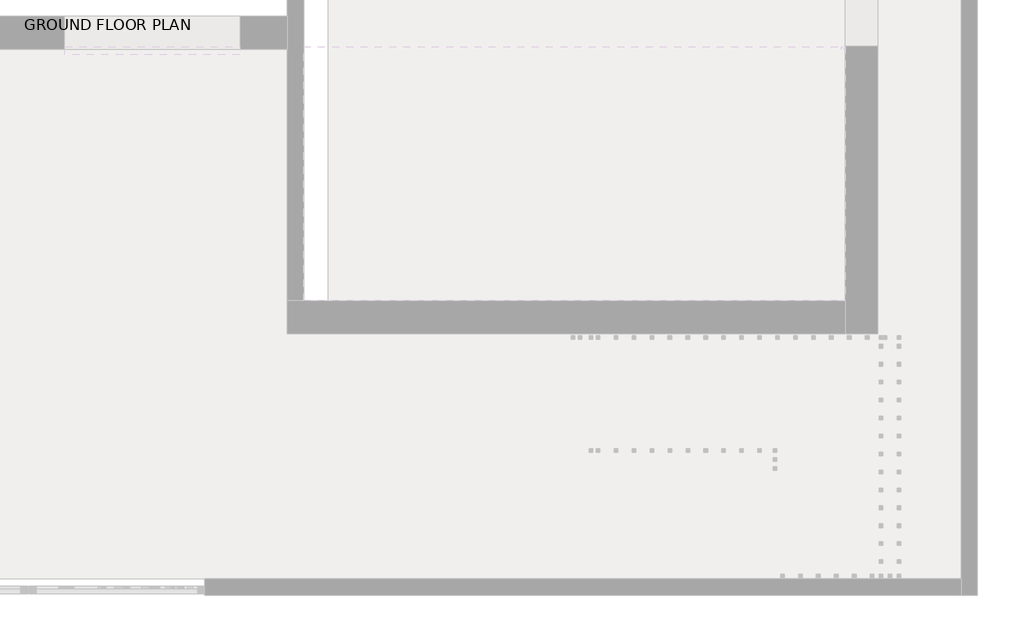
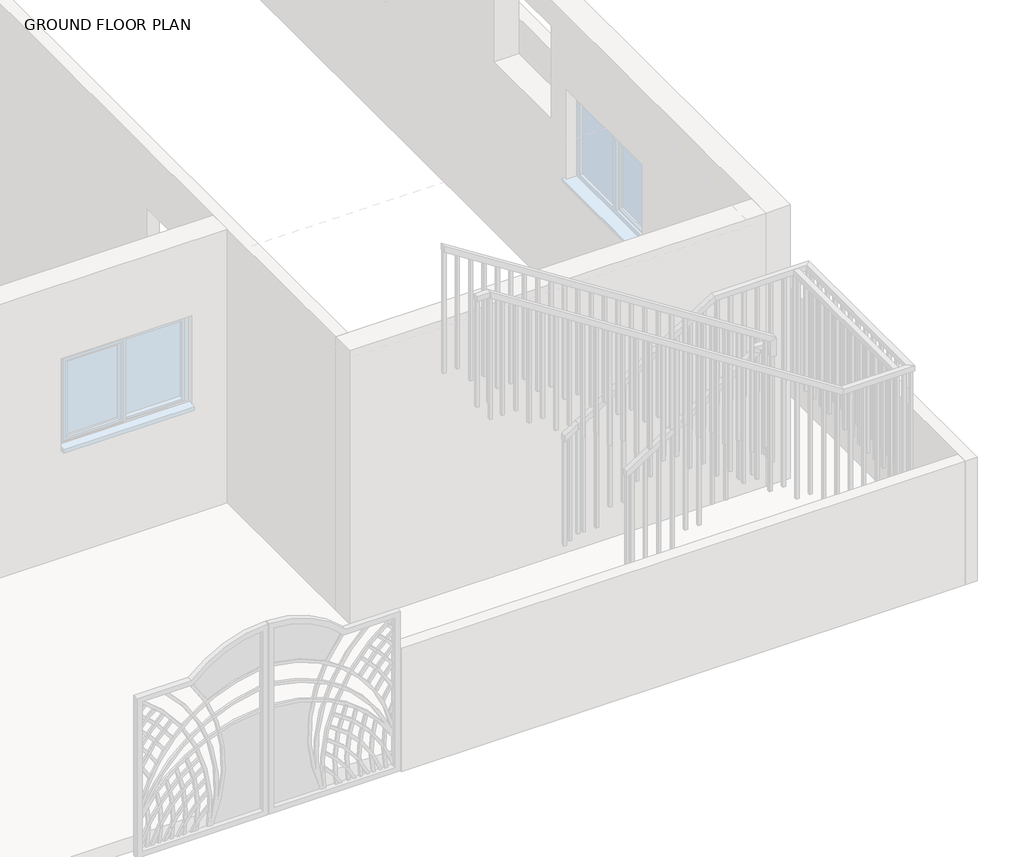
# One storey, part 18 of 23: 2 railings.
"""IFC4 building model written with IfcOpenShell, lengths in millimetres."""

from ifc_helpers import new_model, si_unit, frame, origin, place, context, project, spatial, polyline, outline, extrude, faceted_brep, element, save

model = new_model("IFC4")

# Units and contexts
model_context = context("Model", 3, world=origin())
ifc_project = project(units=[si_unit("LENGTHUNIT", "METRE", prefix="MILLI")], contexts=[model_context])

# Site, building, storey
site = spatial("IfcSite", under=ifc_project)
building = spatial("IfcBuilding", under=site)
storey = spatial("IfcBuildingStorey", under=building, Name="GROUND FLOOR PLAN", Elevation=487.68)

# Railings
placement = place(None, origin())
element("IfcRailing", 1, ObjectType="1100mm", at=placement, inside=storey, context=model_context, shape_type="SolidModel", body=[
    faceted_brep([(-8680.149573, -11007.9255223, 1912.8), (-8680.149573, -11007.9255223, 1853.4423995), (-8680.149573, -11057.9255223, 1853.4423995), (-8680.149573, -11057.9255223, 1912.8), (-7484.3306254, -11007.9255223, 2677.8717446), (-7434.3306254, -11007.9255223, 2650.5035914), (-7434.3306254, -11057.9255223, 2650.5035914), (-7484.3306254, -11057.9255223, 2677.8717446), (-7484.3306254, -11007.9255223, 2725.6), (-7434.3306254, -11007.9255223, 2675.6), (-7434.3306254, -11057.9255223, 2675.6), (-7484.3306254, -11057.9255223, 2725.6), (-7359.3306254, -11007.9255223, 2725.6), (-7359.3306254, -11007.9255223, 2675.6), (-7409.3306254, -11057.9255223, 2675.6), (-7409.3306254, -11057.9255223, 2725.6), (-7359.3306254, -11132.9255223, 2725.6), (-7359.3306254, -11132.9255223, 2675.6), (-7409.3306254, -11132.9255223, 2675.6), (-7409.3306254, -11132.9255223, 2725.6), (-7359.3306254, -11134.9255223, 2725.6), (-7409.3306254, -11134.9255223, 2725.6), (-7409.3306254, -11184.9255223, 2675.6), (-7359.3306254, -11184.9255223, 2675.6)], [[[0, 1, 2, 3]], [[1, 0, 4, 5]], [[2, 1, 5, 6]], [[3, 2, 6, 7]], [[0, 3, 7, 4]], [[5, 4, 8, 9]], [[6, 5, 9, 10]], [[7, 6, 10, 11]], [[4, 7, 11, 8]], [[9, 8, 12, 13]], [[10, 9, 13, 14]], [[11, 10, 14, 15]], [[8, 11, 15, 12]], [[13, 12, 16, 17]], [[14, 13, 17, 18]], [[15, 14, 18, 19]], [[12, 15, 19, 16]], [[20, 21, 22, 23]], [[17, 16, 20, 23]], [[18, 17, 23, 22]], [[19, 18, 22, 21]], [[16, 19, 21, 20]]]),
    faceted_brep([(-7359.3306254, -11184.9255223, 2855.9055527), (-7409.3306254, -11184.9255223, 2828.5415543), (-7409.3306254, -11134.9255223, 2828.5415543), (-7359.3306254, -11134.9255223, 2855.9055527), (-10457.8773536, -11184.9255223, 4838.88), (-10457.8773536, -11134.9255223, 4838.88), (-10457.8773536, -11134.9255223, 4779.517542), (-10457.8773536, -11184.9255223, 4779.517542)], [[[0, 1, 2, 3]], [[4, 5, 6, 7]], [[1, 0, 4, 7]], [[2, 1, 7, 6]], [[3, 2, 6, 5]], [[0, 3, 5, 4]]]),
    faceted_brep([(-7359.3306254, -11134.9255223, 2725.6), (-7359.3306254, -11184.9255223, 2675.6), (-7409.3306254, -11184.9255223, 2675.6), (-7409.3306254, -11134.9255223, 2725.6), (-7359.3306254, -11134.9255223, 2855.9055527), (-7409.3306254, -11134.9255223, 2828.5415543), (-7409.3306254, -11184.9255223, 2828.5415543), (-7359.3306254, -11184.9255223, 2855.9055527)], [[[0, 1, 2, 3]], [[4, 5, 6, 7]], [[1, 0, 4, 7]], [[2, 1, 7, 6]], [[3, 2, 6, 5]], [[0, 3, 5, 4]]]),
    extrude(outline(polyline([(3576.32, -10434.3306254), (4764.4483614, -10434.3306254), (4780.4475912, -10459.3306254), (3576.32, -10459.3306254), (3576.32, -10434.3306254)])), frame((0.0, -11172.4255223, 0.0), z_axis=(0.0, 1.0, 0.0), x_axis=(0.0, 0.0, 1.0)), (0.0, 0.0, 1.0), 25.0),
    extrude(outline(polyline([(3576.32, -10309.3306254), (4684.4522123, -10309.3306254), (4700.4514422, -10334.3306254), (3576.32, -10334.3306254), (3576.32, -10309.3306254)])), frame((0.0, -11172.4255223, 0.0), z_axis=(0.0, 1.0, 0.0), x_axis=(0.0, 0.0, 1.0)), (0.0, 0.0, 1.0), 25.0),
    extrude(outline(polyline([(3413.76, -10184.3306254), (4604.4560633, -10184.3306254), (4620.4552931, -10209.3306254), (3413.76, -10209.3306254), (3413.76, -10184.3306254)])), frame((0.0, -11172.4255223, 0.0), z_axis=(0.0, 1.0, 0.0), x_axis=(0.0, 0.0, 1.0)), (0.0, 0.0, 1.0), 25.0),
    extrude(outline(polyline([(3413.76, -10059.3306254), (4524.4599142, -10059.3306254), (4540.459144, -10084.3306254), (3413.76, -10084.3306254), (3413.76, -10059.3306254)])), frame((0.0, -11172.4255223, 0.0), z_axis=(0.0, 1.0, 0.0), x_axis=(0.0, 0.0, 1.0)), (0.0, 0.0, 1.0), 25.0),
    extrude(outline(polyline([(3251.2, -9934.3306254), (4444.4637652, -9934.3306254), (4460.462995, -9959.3306254), (3251.2, -9959.3306254), (3251.2, -9934.3306254)])), frame((0.0, -11172.4255223, 0.0), z_axis=(0.0, 1.0, 0.0), x_axis=(0.0, 0.0, 1.0)), (0.0, 0.0, 1.0), 25.0),
    extrude(outline(polyline([(3251.2, -9809.3306254), (4364.4676161, -9809.3306254), (4380.4668459, -9834.3306254), (3251.2, -9834.3306254), (3251.2, -9809.3306254)])), frame((0.0, -11172.4255223, 0.0), z_axis=(0.0, 1.0, 0.0), x_axis=(0.0, 0.0, 1.0)), (0.0, 0.0, 1.0), 25.0),
    extrude(outline(polyline([(3251.2, -9684.3306254), (4284.4714671, -9684.3306254), (4300.4706969, -9709.3306254), (3251.2, -9709.3306254), (3251.2, -9684.3306254)])), frame((0.0, -11172.4255223, 0.0), z_axis=(0.0, 1.0, 0.0), x_axis=(0.0, 0.0, 1.0)), (0.0, 0.0, 1.0), 25.0),
    extrude(outline(polyline([(3088.64, -9559.3306254), (4204.475318, -9559.3306254), (4220.4745478, -9584.3306254), (3088.64, -9584.3306254), (3088.64, -9559.3306254)])), frame((0.0, -11172.4255223, 0.0), z_axis=(0.0, 1.0, 0.0), x_axis=(0.0, 0.0, 1.0)), (0.0, 0.0, 1.0), 25.0),
    extrude(outline(polyline([(3088.64, -9434.3306254), (4124.479169, -9434.3306254), (4140.4783988, -9459.3306254), (3088.64, -9459.3306254), (3088.64, -9434.3306254)])), frame((0.0, -11172.4255223, 0.0), z_axis=(0.0, 1.0, 0.0), x_axis=(0.0, 0.0, 1.0)), (0.0, 0.0, 1.0), 25.0),
    extrude(outline(polyline([(2926.08, -9309.3306254), (4044.4830199, -9309.3306254), (4060.4822497, -9334.3306254), (2926.08, -9334.3306254), (2926.08, -9309.3306254)])), frame((0.0, -11172.4255223, 0.0), z_axis=(0.0, 1.0, 0.0), x_axis=(0.0, 0.0, 1.0)), (0.0, 0.0, 1.0), 25.0),
    extrude(outline(polyline([(2926.08, -9184.3306254), (3964.4868709, -9184.3306254), (3980.4861007, -9209.3306254), (2926.08, -9209.3306254), (2926.08, -9184.3306254)])), frame((0.0, -11172.4255223, 0.0), z_axis=(0.0, 1.0, 0.0), x_axis=(0.0, 0.0, 1.0)), (0.0, 0.0, 1.0), 25.0),
    extrude(outline(polyline([(2763.52, -9059.3306254), (3884.4907218, -9059.3306254), (3900.4899516, -9084.3306254), (2763.52, -9084.3306254), (2763.52, -9059.3306254)])), frame((0.0, -11172.4255223, 0.0), z_axis=(0.0, 1.0, 0.0), x_axis=(0.0, 0.0, 1.0)), (0.0, 0.0, 1.0), 25.0),
    extrude(outline(polyline([(2763.52, -8934.3306254), (3804.4945728, -8934.3306254), (3820.4938026, -8959.3306254), (2763.52, -8959.3306254), (2763.52, -8934.3306254)])), frame((0.0, -11172.4255223, 0.0), z_axis=(0.0, 1.0, 0.0), x_axis=(0.0, 0.0, 1.0)), (0.0, 0.0, 1.0), 25.0),
    extrude(outline(polyline([(2600.96, -8809.3306254), (3724.4984237, -8809.3306254), (3740.4976535, -8834.3306254), (2600.96, -8834.3306254), (2600.96, -8809.3306254)])), frame((0.0, -11172.4255223, 0.0), z_axis=(0.0, 1.0, 0.0), x_axis=(0.0, 0.0, 1.0)), (0.0, 0.0, 1.0), 25.0),
    extrude(outline(polyline([(2600.96, -8684.3306254), (3644.5022747, -8684.3306254), (3660.5015045, -8709.3306254), (2600.96, -8709.3306254), (2600.96, -8684.3306254)])), frame((0.0, -11172.4255223, 0.0), z_axis=(0.0, 1.0, 0.0), x_axis=(0.0, 0.0, 1.0)), (0.0, 0.0, 1.0), 25.0),
    extrude(outline(polyline([(2438.4, -8559.3306254), (3564.5061256, -8559.3306254), (3580.5053554, -8584.3306254), (2438.4, -8584.3306254), (2438.4, -8559.3306254)])), frame((0.0, -11172.4255223, 0.0), z_axis=(0.0, 1.0, 0.0), x_axis=(0.0, 0.0, 1.0)), (0.0, 0.0, 1.0), 25.0),
    extrude(outline(polyline([(2438.4, -8434.3306254), (3484.5099766, -8434.3306254), (3500.5092064, -8459.3306254), (2438.4, -8459.3306254), (2438.4, -8434.3306254)])), frame((0.0, -11172.4255223, 0.0), z_axis=(0.0, 1.0, 0.0), x_axis=(0.0, 0.0, 1.0)), (0.0, 0.0, 1.0), 25.0),
    extrude(outline(polyline([(2275.84, -8309.3306254), (3404.5138275, -8309.3306254), (3420.5130573, -8334.3306254), (2275.84, -8334.3306254), (2275.84, -8309.3306254)])), frame((0.0, -11172.4255223, 0.0), z_axis=(0.0, 1.0, 0.0), x_axis=(0.0, 0.0, 1.0)), (0.0, 0.0, 1.0), 25.0),
    extrude(outline(polyline([(2275.84, -8184.3306254), (3324.5176785, -8184.3306254), (3340.5169083, -8209.3306254), (2275.84, -8209.3306254), (2275.84, -8184.3306254)])), frame((0.0, -11172.4255223, 0.0), z_axis=(0.0, 1.0, 0.0), x_axis=(0.0, 0.0, 1.0)), (0.0, 0.0, 1.0), 25.0),
    extrude(outline(polyline([(2113.28, -8059.3306254), (3244.5215294, -8059.3306254), (3260.5207592, -8084.3306254), (2113.28, -8084.3306254), (2113.28, -8059.3306254)])), frame((0.0, -11172.4255223, 0.0), z_axis=(0.0, 1.0, 0.0), x_axis=(0.0, 0.0, 1.0)), (0.0, 0.0, 1.0), 25.0),
    extrude(outline(polyline([(2113.28, -7934.3306254), (3164.5253804, -7934.3306254), (3180.5246102, -7959.3306254), (2113.28, -7959.3306254), (2113.28, -7934.3306254)])), frame((0.0, -11172.4255223, 0.0), z_axis=(0.0, 1.0, 0.0), x_axis=(0.0, 0.0, 1.0)), (0.0, 0.0, 1.0), 25.0),
    extrude(outline(polyline([(1950.72, -7809.3306254), (3084.5292313, -7809.3306254), (3100.5284611, -7834.3306254), (1950.72, -7834.3306254), (1950.72, -7809.3306254)])), frame((0.0, -11172.4255223, 0.0), z_axis=(0.0, 1.0, 0.0), x_axis=(0.0, 0.0, 1.0)), (0.0, 0.0, 1.0), 25.0),
    extrude(outline(polyline([(1950.72, -7684.3306254), (3004.5330823, -7684.3306254), (3020.5323121, -7709.3306254), (1950.72, -7709.3306254), (1950.72, -7684.3306254)])), frame((0.0, -11172.4255223, 0.0), z_axis=(0.0, 1.0, 0.0), x_axis=(0.0, 0.0, 1.0)), (0.0, 0.0, 1.0), 25.0),
    extrude(outline(polyline([(1788.16, -7559.3306254), (2924.5369332, -7559.3306254), (2940.536163, -7584.3306254), (1788.16, -7584.3306254), (1788.16, -7559.3306254)])), frame((0.0, -11172.4255223, 0.0), z_axis=(0.0, 1.0, 0.0), x_axis=(0.0, 0.0, 1.0)), (0.0, 0.0, 1.0), 25.0),
    extrude(outline(polyline([(1788.16, -7434.3306254), (2844.5407841, -7434.3306254), (2860.540014, -7459.3306254), (1788.16, -7459.3306254), (1788.16, -7434.3306254)])), frame((0.0, -11172.4255223, 0.0), z_axis=(0.0, 1.0, 0.0), x_axis=(0.0, 0.0, 1.0)), (0.0, 0.0, 1.0), 25.0),
    extrude(outline(polyline([(-7396.8306254, -11082.9255223), (-7371.8306254, -11082.9255223), (-7371.8306254, -11107.9255223), (-7396.8306254, -11107.9255223), (-7396.8306254, -11082.9255223)])), frame((0.0, 0.0, 1625.6), z_axis=(0.0, 0.0, 1.0), x_axis=(1.0, 0.0, 0.0)), (0.0, 0.0, 1.0), 1050.0),
    extrude(outline(polyline([(2605.1944115, -7505.149573), (1463.04, -7505.149573), (1463.04, -7480.149573), (2621.1891352, -7480.149573), (2605.1944115, -7505.149573)])), frame((0.0, -11045.4255223, 0.0), z_axis=(0.0, 1.0, 0.0), x_axis=(0.0, 0.0, 1.0)), (0.0, 0.0, 1.0), 25.0),
    extrude(outline(polyline([(2525.2207932, -7630.149573), (1463.04, -7630.149573), (1463.04, -7605.149573), (2541.2155169, -7605.149573), (2525.2207932, -7630.149573)])), frame((0.0, -11045.4255223, 0.0), z_axis=(0.0, 1.0, 0.0), x_axis=(0.0, 0.0, 1.0)), (0.0, 0.0, 1.0), 25.0),
    extrude(outline(polyline([(2445.2471749, -7755.149573), (1300.48, -7755.149573), (1300.48, -7730.149573), (2461.2418986, -7730.149573), (2445.2471749, -7755.149573)])), frame((0.0, -11045.4255223, 0.0), z_axis=(0.0, 1.0, 0.0), x_axis=(0.0, 0.0, 1.0)), (0.0, 0.0, 1.0), 25.0),
    extrude(outline(polyline([(2365.2735566, -7880.149573), (1300.48, -7880.149573), (1300.48, -7855.149573), (2381.2682803, -7855.149573), (2365.2735566, -7880.149573)])), frame((0.0, -11045.4255223, 0.0), z_axis=(0.0, 1.0, 0.0), x_axis=(0.0, 0.0, 1.0)), (0.0, 0.0, 1.0), 25.0),
    extrude(outline(polyline([(2285.2999383, -8005.149573), (1137.92, -8005.149573), (1137.92, -7980.149573), (2301.294662, -7980.149573), (2285.2999383, -8005.149573)])), frame((0.0, -11045.4255223, 0.0), z_axis=(0.0, 1.0, 0.0), x_axis=(0.0, 0.0, 1.0)), (0.0, 0.0, 1.0), 25.0),
    extrude(outline(polyline([(2205.32632, -8130.149573), (1137.92, -8130.149573), (1137.92, -8105.149573), (2221.3210437, -8105.149573), (2205.32632, -8130.149573)])), frame((0.0, -11045.4255223, 0.0), z_axis=(0.0, 1.0, 0.0), x_axis=(0.0, 0.0, 1.0)), (0.0, 0.0, 1.0), 25.0),
    extrude(outline(polyline([(2125.3527017, -8255.149573), (975.36, -8255.149573), (975.36, -8230.149573), (2141.3474254, -8230.149573), (2125.3527017, -8255.149573)])), frame((0.0, -11045.4255223, 0.0), z_axis=(0.0, 1.0, 0.0), x_axis=(0.0, 0.0, 1.0)), (0.0, 0.0, 1.0), 25.0),
    extrude(outline(polyline([(2045.3790834, -8380.149573), (975.36, -8380.149573), (975.36, -8355.149573), (2061.3738071, -8355.149573), (2045.3790834, -8380.149573)])), frame((0.0, -11045.4255223, 0.0), z_axis=(0.0, 1.0, 0.0), x_axis=(0.0, 0.0, 1.0)), (0.0, 0.0, 1.0), 25.0),
    extrude(outline(polyline([(1965.4054651, -8505.149573), (812.8, -8505.149573), (812.8, -8480.149573), (1981.4001888, -8480.149573), (1965.4054651, -8505.149573)])), frame((0.0, -11045.4255223, 0.0), z_axis=(0.0, 1.0, 0.0), x_axis=(0.0, 0.0, 1.0)), (0.0, 0.0, 1.0), 25.0),
    extrude(outline(polyline([(1885.4318468, -8630.149573), (812.8, -8630.149573), (812.8, -8605.149573), (1901.4265705, -8605.149573), (1885.4318468, -8630.149573)])), frame((0.0, -11045.4255223, 0.0), z_axis=(0.0, 1.0, 0.0), x_axis=(0.0, 0.0, 1.0)), (0.0, 0.0, 1.0), 25.0),
    extrude(outline(polyline([(-7396.8306254, -11147.4255223), (-7371.8306254, -11147.4255223), (-7371.8306254, -11172.4255223), (-7396.8306254, -11172.4255223), (-7396.8306254, -11147.4255223)])), frame((0.0, 0.0, 1625.6), z_axis=(0.0, 0.0, 1.0), x_axis=(1.0, 0.0, 0.0)), (0.0, 0.0, 1.0), 1050.0),
    extrude(outline(polyline([(-7396.8306254, -11045.4255223), (-7396.8306254, -11020.4255223), (-7371.8306254, -11020.4255223), (-7371.8306254, -11045.4255223), (-7396.8306254, -11045.4255223)])), frame((0.0, 0.0, 1625.6), z_axis=(0.0, 0.0, 1.0), x_axis=(1.0, 0.0, 0.0)), (0.0, 0.0, 1.0), 1050.0),
    extrude(outline(polyline([(3576.32, -10432.8773536), (4763.5183122, -10432.8773536), (4779.517542, -10457.8773536), (3576.32, -10457.8773536), (3576.32, -10432.8773536)])), frame((0.0, -11172.4255223, 0.0), z_axis=(0.0, 1.0, 0.0), x_axis=(0.0, 0.0, 1.0)), (0.0, 0.0, 1.0), 25.0),
    extrude(outline(polyline([(1853.4423995, -8680.149573), (812.8, -8680.149573), (812.8, -8655.149573), (1869.4371231, -8655.149573), (1853.4423995, -8680.149573)])), frame((0.0, -11045.4255223, 0.0), z_axis=(0.0, 1.0, 0.0), x_axis=(0.0, 0.0, 1.0)), (0.0, 0.0, 1.0), 25.0),
])
element("IfcRailing", 2, ObjectType="1100mm", at=placement, inside=storey, context=model_context, shape_type="SolidModel", body=[
    faceted_brep([(-8680.149573, -10220.0521308, 1912.8), (-8680.149573, -10220.0521308, 1853.4423995), (-8680.149573, -10270.0521308, 1853.4423995), (-8680.149573, -10270.0521308, 1912.8), (-7409.7306254, -10220.0521308, 2725.6), (-7395.1045513, -10220.0521308, 2675.6), (-7395.1045513, -10270.0521308, 2675.6), (-7409.7306254, -10270.0521308, 2725.6), (-6495.8132565, -10220.0521308, 2725.6), (-6495.8132565, -10220.0521308, 2675.6), (-6545.8132565, -10270.0521308, 2675.6), (-6545.8132565, -10270.0521308, 2725.6), (-6495.8132565, -11933.6860066, 2725.6), (-6495.8132565, -11933.6860066, 2675.6), (-6545.8132565, -11883.6860066, 2675.6), (-6545.8132565, -11883.6860066, 2725.6), (-7155.718398, -11933.6860066, 2725.6), (-7170.3479429, -11933.6860066, 2675.6), (-7170.3479429, -11883.6860066, 2675.6), (-7155.718398, -11883.6860066, 2725.6), (-10457.8773536, -11933.6860066, 4838.88), (-10457.8773536, -11883.6860066, 4838.88), (-10457.8773536, -11883.6860066, 4779.517542), (-10457.8773536, -11933.6860066, 4779.517542)], [[[0, 1, 2, 3]], [[1, 0, 4, 5]], [[2, 1, 5, 6]], [[3, 2, 6, 7]], [[0, 3, 7, 4]], [[5, 4, 8, 9]], [[6, 5, 9, 10]], [[7, 6, 10, 11]], [[4, 7, 11, 8]], [[9, 8, 12, 13]], [[10, 9, 13, 14]], [[11, 10, 14, 15]], [[8, 11, 15, 12]], [[13, 12, 16, 17]], [[14, 13, 17, 18]], [[15, 14, 18, 19]], [[12, 15, 19, 16]], [[20, 21, 22, 23]], [[17, 16, 20, 23]], [[18, 17, 23, 22]], [[19, 18, 22, 21]], [[16, 19, 21, 20]]]),
    extrude(outline(polyline([(4691.8007425, -10320.8132565), (4707.7999723, -10345.8132565), (3576.32, -10345.8132565), (3576.32, -10320.8132565), (4691.8007425, -10320.8132565)])), frame((0.0, -11921.1860066, 0.0), z_axis=(0.0, 1.0, 0.0), x_axis=(0.0, 0.0, 1.0)), (0.0, 0.0, 1.0), 25.0),
    extrude(outline(polyline([(4611.8045935, -10195.8132565), (4627.8038233, -10220.8132565), (3576.32, -10220.8132565), (3576.32, -10195.8132565), (4611.8045935, -10195.8132565)])), frame((0.0, -11921.1860066, 0.0), z_axis=(0.0, 1.0, 0.0), x_axis=(0.0, 0.0, 1.0)), (0.0, 0.0, 1.0), 25.0),
    extrude(outline(polyline([(4531.8084444, -10070.8132565), (4547.8076742, -10095.8132565), (3413.76, -10095.8132565), (3413.76, -10070.8132565), (4531.8084444, -10070.8132565)])), frame((0.0, -11921.1860066, 0.0), z_axis=(0.0, 1.0, 0.0), x_axis=(0.0, 0.0, 1.0)), (0.0, 0.0, 1.0), 25.0),
    extrude(outline(polyline([(4451.8122954, -9945.8132565), (4467.8115252, -9970.8132565), (3413.76, -9970.8132565), (3413.76, -9945.8132565), (4451.8122954, -9945.8132565)])), frame((0.0, -11921.1860066, 0.0), z_axis=(0.0, 1.0, 0.0), x_axis=(0.0, 0.0, 1.0)), (0.0, 0.0, 1.0), 25.0),
    extrude(outline(polyline([(4371.8161463, -9820.8132565), (4387.8153761, -9845.8132565), (3251.2, -9845.8132565), (3251.2, -9820.8132565), (4371.8161463, -9820.8132565)])), frame((0.0, -11921.1860066, 0.0), z_axis=(0.0, 1.0, 0.0), x_axis=(0.0, 0.0, 1.0)), (0.0, 0.0, 1.0), 25.0),
    extrude(outline(polyline([(4291.8423995, -9695.8132565), (4307.8371231, -9720.8132565), (3251.2, -9720.8132565), (3251.2, -9695.8132565), (4291.8423995, -9695.8132565)])), frame((0.0, -11921.1860066, 0.0), z_axis=(0.0, 1.0, 0.0), x_axis=(0.0, 0.0, 1.0)), (0.0, 0.0, 1.0), 25.0),
    extrude(outline(polyline([(4211.8238482, -9570.8132565), (4227.823078, -9595.8132565), (3088.64, -9595.8132565), (3088.64, -9570.8132565), (4211.8238482, -9570.8132565)])), frame((0.0, -11921.1860066, 0.0), z_axis=(0.0, 1.0, 0.0), x_axis=(0.0, 0.0, 1.0)), (0.0, 0.0, 1.0), 25.0),
    extrude(outline(polyline([(4131.8276992, -9445.8132565), (4147.826929, -9470.8132565), (3088.64, -9470.8132565), (3088.64, -9445.8132565), (4131.8276992, -9445.8132565)])), frame((0.0, -11921.1860066, 0.0), z_axis=(0.0, 1.0, 0.0), x_axis=(0.0, 0.0, 1.0)), (0.0, 0.0, 1.0), 25.0),
    extrude(outline(polyline([(4051.8315501, -9320.8132565), (4067.8307799, -9345.8132565), (2926.08, -9345.8132565), (2926.08, -9320.8132565), (4051.8315501, -9320.8132565)])), frame((0.0, -11921.1860066, 0.0), z_axis=(0.0, 1.0, 0.0), x_axis=(0.0, 0.0, 1.0)), (0.0, 0.0, 1.0), 25.0),
    extrude(outline(polyline([(3971.835401, -9195.8132565), (3987.8346309, -9220.8132565), (2926.08, -9220.8132565), (2926.08, -9195.8132565), (3971.835401, -9195.8132565)])), frame((0.0, -11921.1860066, 0.0), z_axis=(0.0, 1.0, 0.0), x_axis=(0.0, 0.0, 1.0)), (0.0, 0.0, 1.0), 25.0),
    extrude(outline(polyline([(3891.839252, -9070.8132565), (3907.8384818, -9095.8132565), (2763.52, -9095.8132565), (2763.52, -9070.8132565), (3891.839252, -9070.8132565)])), frame((0.0, -11921.1860066, 0.0), z_axis=(0.0, 1.0, 0.0), x_axis=(0.0, 0.0, 1.0)), (0.0, 0.0, 1.0), 25.0),
    extrude(outline(polyline([(3811.8431029, -8945.8132565), (3827.8423328, -8970.8132565), (2763.52, -8970.8132565), (2763.52, -8945.8132565), (3811.8431029, -8945.8132565)])), frame((0.0, -11921.1860066, 0.0), z_axis=(0.0, 1.0, 0.0), x_axis=(0.0, 0.0, 1.0)), (0.0, 0.0, 1.0), 25.0),
    extrude(outline(polyline([(3731.8469539, -8820.8132565), (3747.8461837, -8845.8132565), (2600.96, -8845.8132565), (2600.96, -8820.8132565), (3731.8469539, -8820.8132565)])), frame((0.0, -11921.1860066, 0.0), z_axis=(0.0, 1.0, 0.0), x_axis=(0.0, 0.0, 1.0)), (0.0, 0.0, 1.0), 25.0),
    extrude(outline(polyline([(3651.8508048, -8695.8132565), (3667.8500347, -8720.8132565), (2600.96, -8720.8132565), (2600.96, -8695.8132565), (3651.8508048, -8695.8132565)])), frame((0.0, -11921.1860066, 0.0), z_axis=(0.0, 1.0, 0.0), x_axis=(0.0, 0.0, 1.0)), (0.0, 0.0, 1.0), 25.0),
    extrude(outline(polyline([(3571.8546558, -8570.8132565), (3587.8538856, -8595.8132565), (2438.4, -8595.8132565), (2438.4, -8570.8132565), (3571.8546558, -8570.8132565)])), frame((0.0, -11921.1860066, 0.0), z_axis=(0.0, 1.0, 0.0), x_axis=(0.0, 0.0, 1.0)), (0.0, 0.0, 1.0), 25.0),
    extrude(outline(polyline([(3491.8585067, -8445.8132565), (3507.8577365, -8470.8132565), (2438.4, -8470.8132565), (2438.4, -8445.8132565), (3491.8585067, -8445.8132565)])), frame((0.0, -11921.1860066, 0.0), z_axis=(0.0, 1.0, 0.0), x_axis=(0.0, 0.0, 1.0)), (0.0, 0.0, 1.0), 25.0),
    extrude(outline(polyline([(3411.8623577, -8320.8132565), (3427.8615875, -8345.8132565), (2275.84, -8345.8132565), (2275.84, -8320.8132565), (3411.8623577, -8320.8132565)])), frame((0.0, -11921.1860066, 0.0), z_axis=(0.0, 1.0, 0.0), x_axis=(0.0, 0.0, 1.0)), (0.0, 0.0, 1.0), 25.0),
    extrude(outline(polyline([(3331.8662086, -8195.8132565), (3347.8654384, -8220.8132565), (2275.84, -8220.8132565), (2275.84, -8195.8132565), (3331.8662086, -8195.8132565)])), frame((0.0, -11921.1860066, 0.0), z_axis=(0.0, 1.0, 0.0), x_axis=(0.0, 0.0, 1.0)), (0.0, 0.0, 1.0), 25.0),
    extrude(outline(polyline([(3251.8700596, -8070.8132565), (3267.8692894, -8095.8132565), (2113.28, -8095.8132565), (2113.28, -8070.8132565), (3251.8700596, -8070.8132565)])), frame((0.0, -11921.1860066, 0.0), z_axis=(0.0, 1.0, 0.0), x_axis=(0.0, 0.0, 1.0)), (0.0, 0.0, 1.0), 25.0),
    extrude(outline(polyline([(3171.8739105, -7945.8132565), (3187.8731403, -7970.8132565), (2113.28, -7970.8132565), (2113.28, -7945.8132565), (3171.8739105, -7945.8132565)])), frame((0.0, -11921.1860066, 0.0), z_axis=(0.0, 1.0, 0.0), x_axis=(0.0, 0.0, 1.0)), (0.0, 0.0, 1.0), 25.0),
    extrude(outline(polyline([(3091.8777615, -7820.8132565), (3107.8769913, -7845.8132565), (1950.72, -7845.8132565), (1950.72, -7820.8132565), (3091.8777615, -7820.8132565)])), frame((0.0, -11921.1860066, 0.0), z_axis=(0.0, 1.0, 0.0), x_axis=(0.0, 0.0, 1.0)), (0.0, 0.0, 1.0), 25.0),
    extrude(outline(polyline([(3011.8816124, -7695.8132565), (3027.8808422, -7720.8132565), (1950.72, -7720.8132565), (1950.72, -7695.8132565), (3011.8816124, -7695.8132565)])), frame((0.0, -11921.1860066, 0.0), z_axis=(0.0, 1.0, 0.0), x_axis=(0.0, 0.0, 1.0)), (0.0, 0.0, 1.0), 25.0),
    extrude(outline(polyline([(2931.8854634, -7570.8132565), (2947.8846932, -7595.8132565), (1788.16, -7595.8132565), (1788.16, -7570.8132565), (2931.8854634, -7570.8132565)])), frame((0.0, -11921.1860066, 0.0), z_axis=(0.0, 1.0, 0.0), x_axis=(0.0, 0.0, 1.0)), (0.0, 0.0, 1.0), 25.0),
    extrude(outline(polyline([(2851.8893143, -7445.8132565), (2867.8885441, -7470.8132565), (1788.16, -7470.8132565), (1788.16, -7445.8132565), (2851.8893143, -7445.8132565)])), frame((0.0, -11921.1860066, 0.0), z_axis=(0.0, 1.0, 0.0), x_axis=(0.0, 0.0, 1.0)), (0.0, 0.0, 1.0), 25.0),
    extrude(outline(polyline([(2771.8931653, -7320.8132565), (2787.8923951, -7345.8132565), (1625.6, -7345.8132565), (1625.6, -7320.8132565), (2771.8931653, -7320.8132565)])), frame((0.0, -11921.1860066, 0.0), z_axis=(0.0, 1.0, 0.0), x_axis=(0.0, 0.0, 1.0)), (0.0, 0.0, 1.0), 25.0),
    extrude(outline(polyline([(2691.8970162, -7195.8132565), (2707.896246, -7220.8132565), (1625.6, -7220.8132565), (1625.6, -7195.8132565), (2691.8970162, -7195.8132565)])), frame((0.0, -11921.1860066, 0.0), z_axis=(0.0, 1.0, 0.0), x_axis=(0.0, 0.0, 1.0)), (0.0, 0.0, 1.0), 25.0),
    extrude(outline(polyline([(-7070.8132565, -11921.1860066), (-7095.8132565, -11921.1860066), (-7095.8132565, -11896.1860066), (-7070.8132565, -11896.1860066), (-7070.8132565, -11921.1860066)])), frame((0.0, 0.0, 1625.6), z_axis=(0.0, 0.0, 1.0), x_axis=(1.0, 0.0, 0.0)), (0.0, 0.0, 1.0), 1050.0),
    extrude(outline(polyline([(-6945.8132565, -11921.1860066), (-6970.8132565, -11921.1860066), (-6970.8132565, -11896.1860066), (-6945.8132565, -11896.1860066), (-6945.8132565, -11921.1860066)])), frame((0.0, 0.0, 1625.6), z_axis=(0.0, 0.0, 1.0), x_axis=(1.0, 0.0, 0.0)), (0.0, 0.0, 1.0), 1050.0),
    extrude(outline(polyline([(-6820.8132565, -11921.1860066), (-6845.8132565, -11921.1860066), (-6845.8132565, -11896.1860066), (-6820.8132565, -11896.1860066), (-6820.8132565, -11921.1860066)])), frame((0.0, 0.0, 1625.6), z_axis=(0.0, 0.0, 1.0), x_axis=(1.0, 0.0, 0.0)), (0.0, 0.0, 1.0), 1050.0),
    extrude(outline(polyline([(-6695.8132565, -11921.1860066), (-6720.8132565, -11921.1860066), (-6720.8132565, -11896.1860066), (-6695.8132565, -11896.1860066), (-6695.8132565, -11921.1860066)])), frame((0.0, 0.0, 1625.6), z_axis=(0.0, 0.0, 1.0), x_axis=(1.0, 0.0, 0.0)), (0.0, 0.0, 1.0), 1050.0),
    extrude(outline(polyline([(-6570.8132565, -11921.1860066), (-6595.8132565, -11921.1860066), (-6595.8132565, -11896.1860066), (-6570.8132565, -11896.1860066), (-6570.8132565, -11921.1860066)])), frame((0.0, 0.0, 1625.6), z_axis=(0.0, 0.0, 1.0), x_axis=(1.0, 0.0, 0.0)), (0.0, 0.0, 1.0), 1050.0),
    extrude(outline(polyline([(-6508.3132565, -11795.0521308), (-6508.3132565, -11820.0521308), (-6533.3132565, -11820.0521308), (-6533.3132565, -11795.0521308), (-6508.3132565, -11795.0521308)])), frame((0.0, 0.0, 1625.6), z_axis=(0.0, 0.0, 1.0), x_axis=(1.0, 0.0, 0.0)), (0.0, 0.0, 1.0), 1050.0),
    extrude(outline(polyline([(-6508.3132565, -11670.0521308), (-6508.3132565, -11695.0521308), (-6533.3132565, -11695.0521308), (-6533.3132565, -11670.0521308), (-6508.3132565, -11670.0521308)])), frame((0.0, 0.0, 1625.6), z_axis=(0.0, 0.0, 1.0), x_axis=(1.0, 0.0, 0.0)), (0.0, 0.0, 1.0), 1050.0),
    extrude(outline(polyline([(-6508.3132565, -11545.0521308), (-6508.3132565, -11570.0521308), (-6533.3132565, -11570.0521308), (-6533.3132565, -11545.0521308), (-6508.3132565, -11545.0521308)])), frame((0.0, 0.0, 1625.6), z_axis=(0.0, 0.0, 1.0), x_axis=(1.0, 0.0, 0.0)), (0.0, 0.0, 1.0), 1050.0),
    extrude(outline(polyline([(-6508.3132565, -11420.0521308), (-6508.3132565, -11445.0521308), (-6533.3132565, -11445.0521308), (-6533.3132565, -11420.0521308), (-6508.3132565, -11420.0521308)])), frame((0.0, 0.0, 1625.6), z_axis=(0.0, 0.0, 1.0), x_axis=(1.0, 0.0, 0.0)), (0.0, 0.0, 1.0), 1050.0),
    extrude(outline(polyline([(-6508.3132565, -11295.0521308), (-6508.3132565, -11320.0521308), (-6533.3132565, -11320.0521308), (-6533.3132565, -11295.0521308), (-6508.3132565, -11295.0521308)])), frame((0.0, 0.0, 1625.6), z_axis=(0.0, 0.0, 1.0), x_axis=(1.0, 0.0, 0.0)), (0.0, 0.0, 1.0), 1050.0),
    extrude(outline(polyline([(-6508.3132565, -11170.0521308), (-6508.3132565, -11195.0521308), (-6533.3132565, -11195.0521308), (-6533.3132565, -11170.0521308), (-6508.3132565, -11170.0521308)])), frame((0.0, 0.0, 1625.6), z_axis=(0.0, 0.0, 1.0), x_axis=(1.0, 0.0, 0.0)), (0.0, 0.0, 1.0), 1050.0),
    extrude(outline(polyline([(-6508.3132565, -11045.0521308), (-6508.3132565, -11070.0521308), (-6533.3132565, -11070.0521308), (-6533.3132565, -11045.0521308), (-6508.3132565, -11045.0521308)])), frame((0.0, 0.0, 1625.6), z_axis=(0.0, 0.0, 1.0), x_axis=(1.0, 0.0, 0.0)), (0.0, 0.0, 1.0), 1050.0),
    extrude(outline(polyline([(-6508.3132565, -10920.0521308), (-6508.3132565, -10945.0521308), (-6533.3132565, -10945.0521308), (-6533.3132565, -10920.0521308), (-6508.3132565, -10920.0521308)])), frame((0.0, 0.0, 1625.6), z_axis=(0.0, 0.0, 1.0), x_axis=(1.0, 0.0, 0.0)), (0.0, 0.0, 1.0), 1050.0),
    extrude(outline(polyline([(-6508.3132565, -10795.0521308), (-6508.3132565, -10820.0521308), (-6533.3132565, -10820.0521308), (-6533.3132565, -10795.0521308), (-6508.3132565, -10795.0521308)])), frame((0.0, 0.0, 1625.6), z_axis=(0.0, 0.0, 1.0), x_axis=(1.0, 0.0, 0.0)), (0.0, 0.0, 1.0), 1050.0),
    extrude(outline(polyline([(-6508.3132565, -10670.0521308), (-6508.3132565, -10695.0521308), (-6533.3132565, -10695.0521308), (-6533.3132565, -10670.0521308), (-6508.3132565, -10670.0521308)])), frame((0.0, 0.0, 1625.6), z_axis=(0.0, 0.0, 1.0), x_axis=(1.0, 0.0, 0.0)), (0.0, 0.0, 1.0), 1050.0),
    extrude(outline(polyline([(-6508.3132565, -10545.0521308), (-6508.3132565, -10570.0521308), (-6533.3132565, -10570.0521308), (-6533.3132565, -10545.0521308), (-6508.3132565, -10545.0521308)])), frame((0.0, 0.0, 1625.6), z_axis=(0.0, 0.0, 1.0), x_axis=(1.0, 0.0, 0.0)), (0.0, 0.0, 1.0), 1050.0),
    extrude(outline(polyline([(-6508.3132565, -10420.0521308), (-6508.3132565, -10445.0521308), (-6533.3132565, -10445.0521308), (-6533.3132565, -10420.0521308), (-6508.3132565, -10420.0521308)])), frame((0.0, 0.0, 1625.6), z_axis=(0.0, 0.0, 1.0), x_axis=(1.0, 0.0, 0.0)), (0.0, 0.0, 1.0), 1050.0),
    extrude(outline(polyline([(-6508.3132565, -10295.0521308), (-6508.3132565, -10320.0521308), (-6533.3132565, -10320.0521308), (-6533.3132565, -10295.0521308), (-6508.3132565, -10295.0521308)])), frame((0.0, 0.0, 1625.6), z_axis=(0.0, 0.0, 1.0), x_axis=(1.0, 0.0, 0.0)), (0.0, 0.0, 1.0), 1050.0),
    extrude(outline(polyline([(-6630.149573, -10232.5521308), (-6605.149573, -10232.5521308), (-6605.149573, -10257.5521308), (-6630.149573, -10257.5521308), (-6630.149573, -10232.5521308)])), frame((0.0, 0.0, 1625.6), z_axis=(0.0, 0.0, 1.0), x_axis=(1.0, 0.0, 0.0)), (0.0, 0.0, 1.0), 1050.0),
    extrude(outline(polyline([(-6755.149573, -10232.5521308), (-6730.149573, -10232.5521308), (-6730.149573, -10257.5521308), (-6755.149573, -10257.5521308), (-6755.149573, -10232.5521308)])), frame((0.0, 0.0, 1625.6), z_axis=(0.0, 0.0, 1.0), x_axis=(1.0, 0.0, 0.0)), (0.0, 0.0, 1.0), 1050.0),
    extrude(outline(polyline([(-6880.149573, -10232.5521308), (-6855.149573, -10232.5521308), (-6855.149573, -10257.5521308), (-6880.149573, -10257.5521308), (-6880.149573, -10232.5521308)])), frame((0.0, 0.0, 1625.6), z_axis=(0.0, 0.0, 1.0), x_axis=(1.0, 0.0, 0.0)), (0.0, 0.0, 1.0), 1050.0),
    extrude(outline(polyline([(-7005.149573, -10232.5521308), (-6980.149573, -10232.5521308), (-6980.149573, -10257.5521308), (-7005.149573, -10257.5521308), (-7005.149573, -10232.5521308)])), frame((0.0, 0.0, 1625.6), z_axis=(0.0, 0.0, 1.0), x_axis=(1.0, 0.0, 0.0)), (0.0, 0.0, 1.0), 1050.0),
    extrude(outline(polyline([(-7130.149573, -10232.5521308), (-7105.149573, -10232.5521308), (-7105.149573, -10257.5521308), (-7130.149573, -10257.5521308), (-7130.149573, -10232.5521308)])), frame((0.0, 0.0, 1625.6), z_axis=(0.0, 0.0, 1.0), x_axis=(1.0, 0.0, 0.0)), (0.0, 0.0, 1.0), 1050.0),
    extrude(outline(polyline([(-7255.149573, -10232.5521308), (-7230.149573, -10232.5521308), (-7230.149573, -10257.5521308), (-7255.149573, -10257.5521308), (-7255.149573, -10232.5521308)])), frame((0.0, 0.0, 1625.6), z_axis=(0.0, 0.0, 1.0), x_axis=(1.0, 0.0, 0.0)), (0.0, 0.0, 1.0), 1050.0),
    extrude(outline(polyline([(-7380.149573, -10232.5521308), (-7355.149573, -10232.5521308), (-7355.149573, -10257.5521308), (-7380.149573, -10257.5521308), (-7380.149573, -10232.5521308)])), frame((0.0, 0.0, 1625.6), z_axis=(0.0, 0.0, 1.0), x_axis=(1.0, 0.0, 0.0)), (0.0, 0.0, 1.0), 1050.0),
    extrude(outline(polyline([(1463.04, -7505.149573), (1463.04, -7480.149573), (2621.1891352, -7480.149573), (2605.1944115, -7505.149573), (1463.04, -7505.149573)])), frame((0.0, -10257.5521308, 0.0), z_axis=(0.0, 1.0, 0.0), x_axis=(0.0, 0.0, 1.0)), (0.0, 0.0, 1.0), 25.0),
    extrude(outline(polyline([(1463.04, -7630.149573), (1463.04, -7605.149573), (2541.2155169, -7605.149573), (2525.2207932, -7630.149573), (1463.04, -7630.149573)])), frame((0.0, -10257.5521308, 0.0), z_axis=(0.0, 1.0, 0.0), x_axis=(0.0, 0.0, 1.0)), (0.0, 0.0, 1.0), 25.0),
    extrude(outline(polyline([(1300.48, -7755.149573), (1300.48, -7730.149573), (2461.2418986, -7730.149573), (2445.2471749, -7755.149573), (1300.48, -7755.149573)])), frame((0.0, -10257.5521308, 0.0), z_axis=(0.0, 1.0, 0.0), x_axis=(0.0, 0.0, 1.0)), (0.0, 0.0, 1.0), 25.0),
    extrude(outline(polyline([(1300.48, -7880.149573), (1300.48, -7855.149573), (2381.2682803, -7855.149573), (2365.2735566, -7880.149573), (1300.48, -7880.149573)])), frame((0.0, -10257.5521308, 0.0), z_axis=(0.0, 1.0, 0.0), x_axis=(0.0, 0.0, 1.0)), (0.0, 0.0, 1.0), 25.0),
    extrude(outline(polyline([(1137.92, -8005.149573), (1137.92, -7980.149573), (2301.294662, -7980.149573), (2285.2999383, -8005.149573), (1137.92, -8005.149573)])), frame((0.0, -10257.5521308, 0.0), z_axis=(0.0, 1.0, 0.0), x_axis=(0.0, 0.0, 1.0)), (0.0, 0.0, 1.0), 25.0),
    extrude(outline(polyline([(1137.92, -8130.149573), (1137.92, -8105.149573), (2221.3210437, -8105.149573), (2205.32632, -8130.149573), (1137.92, -8130.149573)])), frame((0.0, -10257.5521308, 0.0), z_axis=(0.0, 1.0, 0.0), x_axis=(0.0, 0.0, 1.0)), (0.0, 0.0, 1.0), 25.0),
    extrude(outline(polyline([(975.36, -8255.149573), (975.36, -8230.149573), (2141.3474254, -8230.149573), (2125.3527017, -8255.149573), (975.36, -8255.149573)])), frame((0.0, -10257.5521308, 0.0), z_axis=(0.0, 1.0, 0.0), x_axis=(0.0, 0.0, 1.0)), (0.0, 0.0, 1.0), 25.0),
    extrude(outline(polyline([(975.36, -8380.149573), (975.36, -8355.149573), (2061.3738071, -8355.149573), (2045.3790834, -8380.149573), (975.36, -8380.149573)])), frame((0.0, -10257.5521308, 0.0), z_axis=(0.0, 1.0, 0.0), x_axis=(0.0, 0.0, 1.0)), (0.0, 0.0, 1.0), 25.0),
    extrude(outline(polyline([(812.8, -8505.149573), (812.8, -8480.149573), (1981.4001888, -8480.149573), (1965.4054651, -8505.149573), (812.8, -8505.149573)])), frame((0.0, -10257.5521308, 0.0), z_axis=(0.0, 1.0, 0.0), x_axis=(0.0, 0.0, 1.0)), (0.0, 0.0, 1.0), 25.0),
    extrude(outline(polyline([(812.8, -8630.149573), (812.8, -8605.149573), (1901.4265705, -8605.149573), (1885.4318468, -8630.149573), (812.8, -8630.149573)])), frame((0.0, -10257.5521308, 0.0), z_axis=(0.0, 1.0, 0.0), x_axis=(0.0, 0.0, 1.0)), (0.0, 0.0, 1.0), 25.0),
    extrude(outline(polyline([(-6508.3132565, -11896.1860066), (-6508.3132565, -11921.1860066), (-6533.3132565, -11921.1860066), (-6533.3132565, -11896.1860066), (-6508.3132565, -11896.1860066)])), frame((0.0, 0.0, 1625.6), z_axis=(0.0, 0.0, 1.0), x_axis=(1.0, 0.0, 0.0)), (0.0, 0.0, 1.0), 1050.0),
    extrude(outline(polyline([(-6533.3132565, -10232.5521308), (-6508.3132565, -10232.5521308), (-6508.3132565, -10257.5521308), (-6533.3132565, -10257.5521308), (-6533.3132565, -10232.5521308)])), frame((0.0, 0.0, 1625.6), z_axis=(0.0, 0.0, 1.0), x_axis=(1.0, 0.0, 0.0)), (0.0, 0.0, 1.0), 1050.0),
    extrude(outline(polyline([(4763.5183122, -10432.8773536), (4779.517542, -10457.8773536), (3576.32, -10457.8773536), (3576.32, -10432.8773536), (4763.5183122, -10432.8773536)])), frame((0.0, -11921.1860066, 0.0), z_axis=(0.0, 1.0, 0.0), x_axis=(0.0, 0.0, 1.0)), (0.0, 0.0, 1.0), 25.0),
    extrude(outline(polyline([(812.8, -8680.149573), (812.8, -8655.149573), (1869.4371231, -8655.149573), (1853.4423995, -8680.149573), (812.8, -8680.149573)])), frame((0.0, -10257.5521308, 0.0), z_axis=(0.0, 1.0, 0.0), x_axis=(0.0, 0.0, 1.0)), (0.0, 0.0, 1.0), 25.0),
])

save(model, "model.ifc")

# Revit data of these elements
# Type "1100mm"
#   built-in parameter 1008612 = 0.019685 (stored number, unit not read)
#   built-in parameter 1008611 = 0.019685 (stored number, unit not read)
#   built-in parameter 1008609 = 0.902231 (stored number, unit not read)
#   built-in parameter 1008604 = 0.19685 (stored number, unit not read)
#   built-in parameter 1008603 = 0.164042 (stored number, unit not read)
#   Railing Height = 3.608924 ft
#   built-in parameter 1008630 = 2
#   built-in parameter 1008610 = 2
#   built-in parameter 1008608 = 1
#   built-in parameter 1008618 = Baluster_Square : 25mm
# Elements 1, 2 (IfcRailing, "1100mm")
#   Phase Created = New Construction
